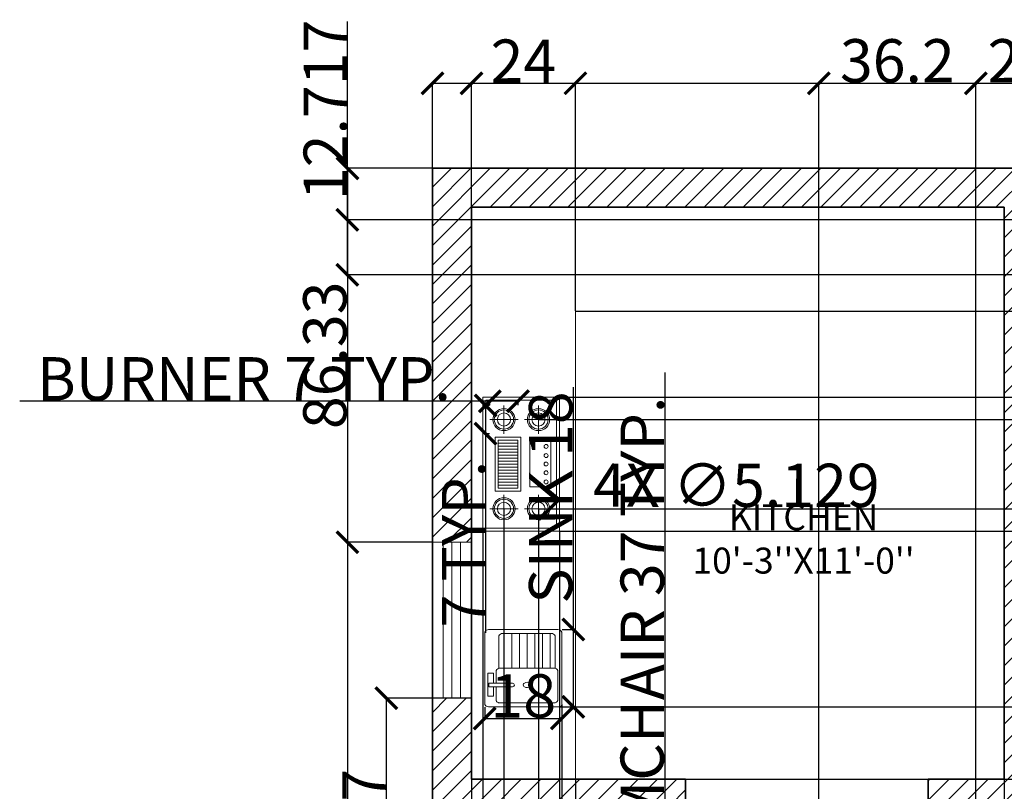
# Model space of a CAD drawing. Units: inches. Extents: x 90933 to 91345, y 21207 to 21646.
# Tile 3 of 4: x 90933 to 91160, y 21458 to 21636. Entities that reach past the tile are written whole.
import ezdxf

# ---------------------------------------------------------------- set-up
doc = ezdxf.new("R2010")
doc.units = ezdxf.units.IN
for name, color, linetype, lineweight in [('A-ANNO-DIMS', 2, 'Continuous', 18), ('A-AREA-IDEN', 7, 'Continuous', 25), ('A-EQPM', 9, 'Continuous', 18), ('A-EQPM-PATT', 9, 'Continuous', 13), ('A-FLOR-CASE', 42, 'Continuous', 18), ('A-FLOR-FIXT', 9, 'Continuous', 18), ('A-WALL-PATT', 8, 'Continuous', 13), ('Walls', 7, 'Continuous', 35), ('Windows', 140, 'Continuous', 18)]:
    doc.layers.add(name, color=color, linetype=linetype, lineweight=lineweight)
doc.styles.get("Standard").update_dxf_attribs({"font": 'arial.ttf'})
doc.dimstyles.get("Standard").update_dxf_attribs({"dimtxt": 10, "dimasz": 5, "dimexe": 0.18, "dimexo": 0.0625, "dimgap": 0.09, "dimtad": 1, "dimdec": 1, "dimzin": 0, "dimdsep": 46, "dimlunit": 4, "dimtxsty": 'Standard', "dimblk": 'ARCHTICK', "dimcen": 0.09, "dimadec": 0, "dimazin": 0, "dimtfac": 1, "dimtdec": 1, "dimtofl": 0, "dimtmove": 0, "dimatfit": 3, "dimldrblk": 'NONE', "dimfxl": 1, "dimtolj": 1, "dimtzin": 0, "dimarcsym": 0})

# ---------------------------------------------------------------- blocks, each defined once
blk = doc.blocks.new('S_SINK12')
for p, q in [((0.25, 0.45), (0.25, 0)), ((0.35, 0.45), (0.35, 0)), ((0.45, 0.45), (0.45, 0)), ((0.55, 0.45), (0.55, 0)), ((0.65, 0.45), (0.65, 0)), ((0.75, 0.45), (0.75, 0)), ((0.85, 0.45), (0.85, 0))]:
    blk.add_line(p, q)
for points in [[(0, -0.469), (0, 0.469, -0.310961), (0.05, 0.5), (0.95, 0.5, -0.310466), (1, 0.469), (1, -0.469, -0.414214), (0.969, -0.5), (0.05, -0.5, -0.309971)], [(0.052, -0.195), (0.052, -0.242), (0.362, -0.242, 1), (0.362, -0.195)], [(0.5, -0.217), (0.503, -0.229, 0.107136), (0.516, -0.241, 0.076468), (0.534, -0.249), (0.554, -0.251), (0.575, -0.248, 0.076468), (0.592, -0.241, 0.107136), (0.604, -0.229), (0.608, -0.217), (0.604, -0.205, 0.107136), (0.592, -0.193, 0.076468), (0.575, -0.186), (0.554, -0.183), (0.532, -0.186, 0.076468), (0.516, -0.193, 0.107136), (0.503, -0.205)]]:
    blk.add_lwpolyline(points, format="xyb", close=True)
for points in [[(0.185, -0.001), (0.185, 0.419, -0.310466), (0.235, 0.45), (0.862, 0.45, -0.310466), (0.912, 0.419), (0.912, 0, -0.310466)], [(0.15, -0.195), (0.15, -0.031, -0.310466), (0.2, 0), (0.9, 0, -0.310466), (0.95, -0.031), (0.95, -0.419, -0.310466), (0.9, -0.45), (0.2, -0.45), (0.18, -0.448, -0.071009), (0.165, -0.442, -0.106323), (0.153, -0.432), (0.15, -0.422), (0.151, -0.419)]]:
    blk.add_lwpolyline(points, format="xyb")
for points in [[(0.114, -0.242), (0.114, -0.364), (0.039, -0.364), (0.039, -0.064), (0.114, -0.064), (0.114, -0.195)], [(0.15, -0.419), (0.15, -0.242)]]:
    blk.add_lwpolyline(points)
blk = doc.blocks.new('COOKTOP-BURNER')
for p, q in [((0, -3.26), (0, 3.26)), ((3.26, 0), (-3.26, 0))]:
    blk.add_line(p, q)
for radius in [2.56, 2.22, 1.52]:
    blk.add_circle((0, 0), radius)
blk = doc.blocks.new('WINDOW-GLAZING-36IN')
for p, q in [((0, 4), (36, 4)), ((0, 2), (36, 2)), ((0, 0), (36, 0))]:
    blk.add_line(p, q)
blk = doc.blocks.new('_ArchTick')
at = {"color": 0, "linetype": 'ByBlock', "const_width": 0.15}
blk.add_lwpolyline([(-0.5, -0.5), (0.5, 0.5)], dxfattribs=at)
blk = doc.blocks.new('*D18')
at = {"layer": 'A-ANNO-DIMS', "color": 0, "lineweight": -2, "transparency": 16777216}
for p, q in [((91041.35, 21547.85), (90932.83, 21547.85)), ((91041.35, 21546.93), (91041.35, 21548.03)), ((91047.87, 21547.85), (91041.35, 21547.85)), ((91047.87, 21546.93), (91047.87, 21548.03))]:
    blk.add_line(p, q, dxfattribs=at)
at = {"layer": 'Defpoints', "color": 0, "transparency": 16777216}
for p in [(91041.35, 21547.85), (91041.35, 21546.87), (91047.87, 21546.87)]:
    blk.add_point(p, dxfattribs=at)
at = {"layer": 'A-ANNO-DIMS', "color": 0, "lineweight": -2, "transparency": 16777216, "xscale": 5, "yscale": 5, "zscale": 5, "rotation": 180}
blk.add_blockref('_ArchTick', (91041.35, 21547.85), dxfattribs=at)
at = {"layer": 'A-ANNO-DIMS', "color": 0, "lineweight": -2, "transparency": 16777216, "xscale": 5, "yscale": 5, "zscale": 5}
blk.add_blockref('_ArchTick', (91047.87, 21547.85), dxfattribs=at)
at = {"layer": 'A-ANNO-DIMS', "color": 0, "transparency": 16777216, "insert": (90984.59, 21553.02), "char_height": 10, "attachment_point": 5}
blk.add_mtext('\\A1;BURNER 7 TYP.', dxfattribs=at)
blk = doc.blocks.new('_None')
blk = doc.blocks.new('*D19')
at = {"layer": 'A-ANNO-DIMS', "color": 0, "lineweight": -2, "transparency": 16777216}
for p, q in [((91041.29, 21546.87), (91040.19, 21546.87)), ((91040.37, 21546.87), (91040.37, 21540.35)), ((91041.29, 21540.35), (91040.19, 21540.35)), ((91040.37, 21540.35), (91040.37, 21494.35))]:
    blk.add_line(p, q, dxfattribs=at)
at = {"layer": 'Defpoints', "color": 0, "transparency": 16777216}
for p in [(91041.35, 21546.87), (91040.37, 21540.35), (91041.35, 21540.35)]:
    blk.add_point(p, dxfattribs=at)
at = {"layer": 'A-ANNO-DIMS', "color": 0, "lineweight": -2, "transparency": 16777216, "xscale": 5, "yscale": 5, "zscale": 5}
for p, rotation in [((91040.37, 21546.87), 90), ((91040.37, 21540.35), 270)]:
    blk.add_blockref('_ArchTick', p, dxfattribs=dict(at, rotation=rotation))
at = {"layer": 'A-ANNO-DIMS', "color": 0, "transparency": 16777216, "insert": (91035.28, 21514.85), "char_height": 10, "attachment_point": 5, "rotation": 90}
blk.add_mtext('\\A1;7 TYP.', dxfattribs=at)
blk = doc.blocks.new('*D24')
at = {"layer": 'A-ANNO-DIMS', "color": 0, "lineweight": -2, "transparency": 16777216}
for p, q in [((91081.79, 21421.63), (91081.79, 21554.45)), ((91076.29, 21421.63), (91081.97, 21421.63)), ((91081.79, 21384.54), (91081.79, 21421.63)), ((91076.29, 21384.54), (91081.97, 21384.54))]:
    blk.add_line(p, q, dxfattribs=at)
at = {"layer": 'Defpoints', "color": 0, "transparency": 16777216}
for p in [(91076.22, 21421.63), (91081.79, 21421.63), (91076.22, 21384.54)]:
    blk.add_point(p, dxfattribs=at)
at = {"layer": 'A-ANNO-DIMS', "color": 0, "lineweight": -2, "transparency": 16777216, "xscale": 5, "yscale": 5, "zscale": 5}
for p, rotation in [((91081.79, 21421.63), 90), ((91081.79, 21384.54), 270)]:
    blk.add_blockref('_ArchTick', p, dxfattribs=dict(at, rotation=rotation))
at = {"layer": 'A-ANNO-DIMS', "color": 0, "transparency": 16777216, "insert": (91076.52, 21490.54), "char_height": 10, "attachment_point": 5, "rotation": 90}
blk.add_mtext('\\A1;ARMCHAIR 37 TYP.', dxfattribs=at)
blk = doc.blocks.new('*D34')
at = {"layer": 'A-ANNO-DIMS', "color": 0, "lineweight": -2, "transparency": 16777216}
for p, q in [((91060.64, 21495.13), (91060.64, 21551.09)), ((91058.03, 21495.13), (91060.82, 21495.13)), ((91060.64, 21477.3), (91060.64, 21495.13)), ((91058.03, 21477.3), (91060.82, 21477.3))]:
    blk.add_line(p, q, dxfattribs=at)
at = {"layer": 'Defpoints', "color": 0, "transparency": 16777216}
for p in [(91057.97, 21495.13), (91060.64, 21495.13), (91057.97, 21477.3)]:
    blk.add_point(p, dxfattribs=at)
at = {"layer": 'A-ANNO-DIMS', "color": 0, "lineweight": -2, "transparency": 16777216, "xscale": 5, "yscale": 5, "zscale": 5}
for p, rotation in [((91060.64, 21495.13), 90), ((91060.64, 21477.3), 270)]:
    blk.add_blockref('_ArchTick', p, dxfattribs=dict(at, rotation=rotation))
at = {"layer": 'A-ANNO-DIMS', "color": 0, "transparency": 16777216, "insert": (91055.38, 21525.61), "char_height": 10, "attachment_point": 5, "rotation": 90}
blk.add_mtext('\\A1;SINK 18', dxfattribs=at)
blk = doc.blocks.new('*D35')
at = {"layer": 'A-ANNO-DIMS', "color": 0, "lineweight": -2, "transparency": 16777216}
for p, q in [((91040.17, 21477.23), (91040.17, 21474.44)), ((91057.97, 21477.23), (91057.97, 21474.44)), ((91040.17, 21474.62), (91057.97, 21474.62))]:
    blk.add_line(p, q, dxfattribs=at)
at = {"layer": 'Defpoints', "color": 0, "transparency": 16777216}
for p in [(91040.17, 21477.3), (91057.97, 21477.3), (91057.97, 21474.62)]:
    blk.add_point(p, dxfattribs=at)
at = {"layer": 'A-ANNO-DIMS', "color": 0, "lineweight": -2, "transparency": 16777216, "xscale": 5, "yscale": 5, "zscale": 5, "rotation": 180}
blk.add_blockref('_ArchTick', (91040.17, 21474.62), dxfattribs=at)
at = {"layer": 'A-ANNO-DIMS', "color": 0, "lineweight": -2, "transparency": 16777216, "xscale": 5, "yscale": 5, "zscale": 5}
blk.add_blockref('_ArchTick', (91057.97, 21474.62), dxfattribs=at)
at = {"layer": 'A-ANNO-DIMS', "color": 0, "transparency": 16777216, "insert": (91049.07, 21479.82), "char_height": 10, "attachment_point": 5}
blk.add_mtext('\\A1;18', dxfattribs=at)
blk = doc.blocks.new('*D42')
at = {"layer": 'A-ANNO-DIMS', "color": 0, "lineweight": -2, "transparency": 16777216}
for p, q in [((91028.04, 21601.62), (91008.29, 21601.62)), ((91008.47, 21601.62), (91008.47, 21515.28)), ((91028.04, 21515.28), (91008.29, 21515.28))]:
    blk.add_line(p, q, dxfattribs=at)
at = {"layer": 'Defpoints', "color": 0, "transparency": 16777216}
for p in [(91028.1, 21601.62), (91008.47, 21515.28), (91028.1, 21515.28)]:
    blk.add_point(p, dxfattribs=at)
at = {"layer": 'A-ANNO-DIMS', "color": 0, "lineweight": -2, "transparency": 16777216, "xscale": 5, "yscale": 5, "zscale": 5}
for p, rotation in [((91008.47, 21601.62), 90), ((91008.47, 21515.28), 270)]:
    blk.add_blockref('_ArchTick', p, dxfattribs=dict(at, rotation=rotation))
at = {"layer": 'A-ANNO-DIMS', "color": 0, "transparency": 16777216, "insert": (91003.27, 21558.45), "char_height": 10, "attachment_point": 5, "rotation": 90}
blk.add_mtext('\\A1;86.33', dxfattribs=at)
blk = doc.blocks.new('*D43')
at = {"layer": 'A-ANNO-DIMS', "color": 0, "lineweight": -2, "transparency": 16777216}
for p, q in [((91037.04, 21479.28), (91017.29, 21479.28)), ((91017.47, 21412.62), (91017.47, 21479.28)), ((91037.04, 21412.62), (91017.29, 21412.62))]:
    blk.add_line(p, q, dxfattribs=at)
at = {"layer": 'Defpoints', "color": 0, "transparency": 16777216}
for p in [(91017.47, 21479.28), (91037.1, 21479.28), (91037.1, 21412.62)]:
    blk.add_point(p, dxfattribs=at)
at = {"layer": 'A-ANNO-DIMS', "color": 0, "lineweight": -2, "transparency": 16777216, "xscale": 5, "yscale": 5, "zscale": 5}
for p, rotation in [((91017.47, 21479.28), 90), ((91017.47, 21412.62), 270)]:
    blk.add_blockref('_ArchTick', p, dxfattribs=dict(at, rotation=rotation))
at = {"layer": 'A-ANNO-DIMS', "color": 0, "transparency": 16777216, "insert": (91012.27, 21445.95), "char_height": 10, "attachment_point": 5, "rotation": 90}
blk.add_mtext('\\A1;66.67', dxfattribs=at)
blk = doc.blocks.new('*D49')
at = {"layer": 'A-ANNO-DIMS', "color": 0, "lineweight": -2, "transparency": 16777216}
for p, q in [((91160.1, 21460.55), (91160.1, 21209.81)), ((91142.5, 21454.55), (91142.5, 21209.81)), ((91142.5, 21209.99), (91160.1, 21209.99)), ((91160.1, 21209.99), (91205.85, 21209.99))]:
    blk.add_line(p, q, dxfattribs=at)
at = {"layer": 'Defpoints', "color": 0, "transparency": 16777216}
for p in [(91160.1, 21460.62), (91142.5, 21454.62), (91160.1, 21209.99)]:
    blk.add_point(p, dxfattribs=at)
at = {"layer": 'A-ANNO-DIMS', "color": 0, "lineweight": -2, "transparency": 16777216, "xscale": 5, "yscale": 5, "zscale": 5, "rotation": 180}
blk.add_blockref('_ArchTick', (91142.5, 21209.99), dxfattribs=at)
at = {"layer": 'A-ANNO-DIMS', "color": 0, "lineweight": -2, "transparency": 16777216, "xscale": 5, "yscale": 5, "zscale": 5}
blk.add_blockref('_ArchTick', (91160.1, 21209.99), dxfattribs=at)
at = {"layer": 'A-ANNO-DIMS', "color": 0, "transparency": 16777216, "insert": (91185.47, 21215.18), "char_height": 10, "attachment_point": 5}
blk.add_mtext('\\A1;17.596', dxfattribs=at)
blk = doc.blocks.new('*D52')
at = {"layer": 'A-ANNO-DIMS', "color": 0, "lineweight": -2, "transparency": 16777216}
for p, q in [((91037.1, 21592.68), (91037.1, 21621.43)), ((91037.1, 21621.25), (91061.1, 21621.25)), ((91061.1, 21568.68), (91061.1, 21621.43))]:
    blk.add_line(p, q, dxfattribs=at)
at = {"layer": 'Defpoints', "color": 0, "transparency": 16777216}
for p in [(91061.1, 21621.25), (91037.1, 21592.62), (91061.1, 21568.62)]:
    blk.add_point(p, dxfattribs=at)
at = {"layer": 'A-ANNO-DIMS', "color": 0, "lineweight": -2, "transparency": 16777216, "xscale": 5, "yscale": 5, "zscale": 5, "rotation": 180}
blk.add_blockref('_ArchTick', (91037.1, 21621.25), dxfattribs=at)
at = {"layer": 'A-ANNO-DIMS', "color": 0, "lineweight": -2, "transparency": 16777216, "xscale": 5, "yscale": 5, "zscale": 5}
blk.add_blockref('_ArchTick', (91061.1, 21621.25), dxfattribs=at)
at = {"layer": 'A-ANNO-DIMS', "color": 0, "transparency": 16777216, "insert": (91049.1, 21626.36), "char_height": 10, "attachment_point": 5}
blk.add_mtext('\\A1;24', dxfattribs=at)
blk = doc.blocks.new('*D53')
at = {"layer": 'A-ANNO-DIMS', "color": 0, "lineweight": -2, "transparency": 16777216}
for p, q in [((91160.1, 21460.55), (91160.1, 21209.81)), ((91166.1, 21460.55), (91166.1, 21209.81)), ((91160.1, 21209.99), (91166.1, 21209.99)), ((91166.1, 21209.99), (91177.88, 21209.99))]:
    blk.add_line(p, q, dxfattribs=at)
at = {"layer": 'Defpoints', "color": 0, "transparency": 16777216}
for p in [(91160.1, 21460.62), (91166.1, 21460.62), (91166.1, 21209.99)]:
    blk.add_point(p, dxfattribs=at)
at = {"layer": 'A-ANNO-DIMS', "color": 0, "lineweight": -2, "transparency": 16777216, "xscale": 5, "yscale": 5, "zscale": 5, "rotation": 180}
blk.add_blockref('_ArchTick', (91160.1, 21209.99), dxfattribs=at)
at = {"layer": 'A-ANNO-DIMS', "color": 0, "lineweight": -2, "transparency": 16777216, "xscale": 5, "yscale": 5, "zscale": 5}
blk.add_blockref('_ArchTick', (91166.1, 21209.99), dxfattribs=at)
at = {"layer": 'A-ANNO-DIMS', "color": 0, "transparency": 16777216, "insert": (91174.49, 21215.18), "char_height": 10, "attachment_point": 5}
blk.add_mtext('\\A1;6', dxfattribs=at)
blk = doc.blocks.new('*D58')
at = {"layer": 'A-ANNO-DIMS', "color": 0, "lineweight": -2, "transparency": 16777216}
for p, q in [((91039.71, 21517.79), (91039.71, 21209.81)), ((91057.43, 21517.79), (91057.43, 21209.81)), ((91039.71, 21209.99), (91057.43, 21209.99)), ((91057.43, 21209.99), (91103.17, 21209.99))]:
    blk.add_line(p, q, dxfattribs=at)
at = {"layer": 'Defpoints', "color": 0, "transparency": 16777216}
for p in [(91039.71, 21517.85), (91057.43, 21517.85), (91057.43, 21209.99)]:
    blk.add_point(p, dxfattribs=at)
at = {"layer": 'A-ANNO-DIMS', "color": 0, "lineweight": -2, "transparency": 16777216, "xscale": 5, "yscale": 5, "zscale": 5, "rotation": 180}
blk.add_blockref('_ArchTick', (91039.71, 21209.99), dxfattribs=at)
at = {"layer": 'A-ANNO-DIMS', "color": 0, "lineweight": -2, "transparency": 16777216, "xscale": 5, "yscale": 5, "zscale": 5}
blk.add_blockref('_ArchTick', (91057.43, 21209.99), dxfattribs=at)
at = {"layer": 'A-ANNO-DIMS', "color": 0, "transparency": 16777216, "insert": (91082.8, 21215.18), "char_height": 10, "attachment_point": 5}
blk.add_mtext('\\A1;17.716', dxfattribs=at)
blk = doc.blocks.new('*D59')
at = {"layer": 'A-ANNO-DIMS', "color": 0, "lineweight": -2, "transparency": 16777216}
for p, q in [((91326.73, 21548.77), (91326.73, 21595.45)), ((91057.49, 21548.77), (91326.91, 21548.77)), ((91326.73, 21517.85), (91326.73, 21548.77)), ((91057.49, 21517.85), (91326.91, 21517.85))]:
    blk.add_line(p, q, dxfattribs=at)
at = {"layer": 'Defpoints', "color": 0, "transparency": 16777216}
for p in [(91057.43, 21548.77), (91326.73, 21548.77), (91057.43, 21517.85)]:
    blk.add_point(p, dxfattribs=at)
at = {"layer": 'A-ANNO-DIMS', "color": 0, "lineweight": -2, "transparency": 16777216, "xscale": 5, "yscale": 5, "zscale": 5}
for p, rotation in [((91326.73, 21548.77), 90), ((91326.73, 21517.85), 270)]:
    blk.add_blockref('_ArchTick', p, dxfattribs=dict(at, rotation=rotation))
at = {"layer": 'A-ANNO-DIMS', "color": 0, "transparency": 16777216, "insert": (91321.53, 21574.61), "char_height": 10, "attachment_point": 5, "rotation": 90}
blk.add_mtext('\\A1;30.916', dxfattribs=at)
blk = doc.blocks.new('*D60')
at = {"layer": 'A-ANNO-DIMS', "color": 0, "lineweight": -2, "transparency": 16777216}
for p, q in [((91117.31, 21395.74), (91117.31, 21621.43)), ((91117.31, 21621.25), (91153.51, 21621.25)), ((91153.51, 21395.74), (91153.51, 21621.43))]:
    blk.add_line(p, q, dxfattribs=at)
at = {"layer": 'Defpoints', "color": 0, "transparency": 16777216}
for p in [(91153.51, 21621.25), (91117.31, 21395.68), (91153.51, 21395.68)]:
    blk.add_point(p, dxfattribs=at)
at = {"layer": 'A-ANNO-DIMS', "color": 0, "lineweight": -2, "transparency": 16777216, "xscale": 5, "yscale": 5, "zscale": 5, "rotation": 180}
blk.add_blockref('_ArchTick', (91117.31, 21621.25), dxfattribs=at)
at = {"layer": 'A-ANNO-DIMS', "color": 0, "lineweight": -2, "transparency": 16777216, "xscale": 5, "yscale": 5, "zscale": 5}
blk.add_blockref('_ArchTick', (91153.51, 21621.25), dxfattribs=at)
at = {"layer": 'A-ANNO-DIMS', "color": 0, "transparency": 16777216, "insert": (91135.41, 21626.44), "char_height": 10, "attachment_point": 5}
blk.add_mtext('\\A1;36.2', dxfattribs=at)
blk = doc.blocks.new('*D63')
at = {"layer": 'A-ANNO-DIMS', "color": 0, "lineweight": -2, "transparency": 16777216}
for p, q in [((91008.47, 21589.73), (91008.47, 21635.49)), ((91252.43, 21589.73), (91008.29, 21589.73)), ((91008.47, 21577.01), (91008.47, 21589.73)), ((91252.43, 21577.01), (91008.29, 21577.01))]:
    blk.add_line(p, q, dxfattribs=at)
at = {"layer": 'Defpoints', "color": 0, "transparency": 16777216}
for p in [(91008.47, 21589.73), (91252.49, 21589.73), (91252.49, 21577.01)]:
    blk.add_point(p, dxfattribs=at)
at = {"layer": 'A-ANNO-DIMS', "color": 0, "lineweight": -2, "transparency": 16777216, "xscale": 5, "yscale": 5, "zscale": 5}
for p, rotation in [((91008.47, 21589.73), 90), ((91008.47, 21577.01), 270)]:
    blk.add_blockref('_ArchTick', p, dxfattribs=dict(at, rotation=rotation))
at = {"layer": 'A-ANNO-DIMS', "color": 0, "transparency": 16777216, "insert": (91003.36, 21615.11), "char_height": 10, "attachment_point": 5, "rotation": 90}
blk.add_mtext('\\A1;12.717', dxfattribs=at)
blk = doc.blocks.new('*D64')
at = {"layer": 'A-ANNO-DIMS', "color": 0, "lineweight": -2, "transparency": 16777216}
for p, q in [((91028.1, 21601.68), (91028.1, 21621.43)), ((91028.1, 21621.25), (91307.1, 21621.25)), ((91307.1, 21601.68), (91307.1, 21621.43))]:
    blk.add_line(p, q, dxfattribs=at)
at = {"layer": 'Defpoints', "color": 0, "transparency": 16777216}
for p in [(91307.1, 21621.25), (91028.1, 21601.62), (91307.1, 21601.62)]:
    blk.add_point(p, dxfattribs=at)
at = {"layer": 'A-ANNO-DIMS', "color": 0, "lineweight": -2, "transparency": 16777216, "xscale": 5, "yscale": 5, "zscale": 5, "rotation": 180}
blk.add_blockref('_ArchTick', (91028.1, 21621.25), dxfattribs=at)
at = {"layer": 'A-ANNO-DIMS', "color": 0, "lineweight": -2, "transparency": 16777216, "xscale": 5, "yscale": 5, "zscale": 5}
blk.add_blockref('_ArchTick', (91307.1, 21621.25), dxfattribs=at)
at = {"layer": 'A-ANNO-DIMS', "color": 0, "transparency": 16777216, "insert": (91167.6, 21626.44), "char_height": 10, "attachment_point": 5}
blk.add_mtext('\\A1;279', dxfattribs=at)
blk = doc.blocks.new('*D65')
at = {"layer": 'A-ANNO-DIMS', "color": 0, "lineweight": -2, "transparency": 16777216}
for p, q in [((91028.04, 21601.62), (91008.29, 21601.62)), ((91008.47, 21601.62), (91008.47, 21229.62)), ((91028.04, 21229.62), (91008.29, 21229.62))]:
    blk.add_line(p, q, dxfattribs=at)
at = {"layer": 'Defpoints', "color": 0, "transparency": 16777216}
for p in [(91028.1, 21601.62), (91008.47, 21229.62), (91028.1, 21229.62)]:
    blk.add_point(p, dxfattribs=at)
at = {"layer": 'A-ANNO-DIMS', "color": 0, "lineweight": -2, "transparency": 16777216, "xscale": 5, "yscale": 5, "zscale": 5}
for p, rotation in [((91008.47, 21601.62), 90), ((91008.47, 21229.62), 270)]:
    blk.add_blockref('_ArchTick', p, dxfattribs=dict(at, rotation=rotation))
at = {"layer": 'A-ANNO-DIMS', "color": 0, "transparency": 16777216, "insert": (91003.27, 21415.62), "char_height": 10, "attachment_point": 5, "rotation": 90}
blk.add_mtext('\\A1;372', dxfattribs=at)
blk = doc.blocks.new('*D66')
at = {"layer": 'A-ANNO-DIMS', "color": 0, "lineweight": -2, "transparency": 16777216}
for p, q in [((91061.16, 21568.62), (91326.91, 21568.62)), ((91326.73, 21568.62), (91326.73, 21548.77)), ((91057.49, 21548.77), (91326.91, 21548.77)), ((91326.73, 21548.77), (91326.73, 21503.02))]:
    blk.add_line(p, q, dxfattribs=at)
at = {"layer": 'Defpoints', "color": 0, "transparency": 16777216}
for p in [(91061.1, 21568.62), (91057.43, 21548.77), (91326.73, 21548.77)]:
    blk.add_point(p, dxfattribs=at)
at = {"layer": 'A-ANNO-DIMS', "color": 0, "lineweight": -2, "transparency": 16777216, "xscale": 5, "yscale": 5, "zscale": 5}
for p, rotation in [((91326.73, 21568.62), 90), ((91326.73, 21548.77), 270)]:
    blk.add_blockref('_ArchTick', p, dxfattribs=dict(at, rotation=rotation))
at = {"layer": 'A-ANNO-DIMS', "color": 0, "transparency": 16777216, "insert": (91321.53, 21523.4), "char_height": 10, "attachment_point": 5, "rotation": 90}
blk.add_mtext('\\A1;19.846', dxfattribs=at)
blk = doc.blocks.new('*D67')
at = {"layer": 'A-ANNO-DIMS', "color": 0, "lineweight": -2, "transparency": 16777216}
for p, q in [((91326.73, 21477.31), (91326.73, 21507.53)), ((91057.47, 21477.31), (91326.91, 21477.31)), ((91326.73, 21460.62), (91326.73, 21477.31)), ((91061.16, 21460.62), (91326.91, 21460.62))]:
    blk.add_line(p, q, dxfattribs=at)
at = {"layer": 'Defpoints', "color": 0, "transparency": 16777216}
for p in [(91057.41, 21477.31), (91326.73, 21477.31), (91061.1, 21460.62)]:
    blk.add_point(p, dxfattribs=at)
at = {"layer": 'A-ANNO-DIMS', "color": 0, "lineweight": -2, "transparency": 16777216, "xscale": 5, "yscale": 5, "zscale": 5}
for p, rotation in [((91326.73, 21477.31), 90), ((91326.73, 21460.62), 270)]:
    blk.add_blockref('_ArchTick', p, dxfattribs=dict(at, rotation=rotation))
at = {"layer": 'A-ANNO-DIMS', "color": 0, "transparency": 16777216, "insert": (91321.53, 21494.92), "char_height": 10, "attachment_point": 5, "rotation": 90}
blk.add_mtext('\\A1;16.7', dxfattribs=at)
blk = doc.blocks.new('*D71')
at = {"layer": 'A-ANNO-DIMS', "color": 0, "lineweight": -2, "transparency": 16777216}
for p, q in [((91044.61, 21522.95), (91044.61, 21209.81)), ((91052.59, 21522.95), (91052.59, 21209.81)), ((91044.61, 21209.99), (91052.59, 21209.99)), ((91052.59, 21209.99), (91083.68, 21209.99))]:
    blk.add_line(p, q, dxfattribs=at)
at = {"layer": 'Defpoints', "color": 0, "transparency": 16777216}
for p in [(91044.61, 21523.01), (91052.59, 21523.01), (91052.59, 21209.99)]:
    blk.add_point(p, dxfattribs=at)
at = {"layer": 'A-ANNO-DIMS', "color": 0, "lineweight": -2, "transparency": 16777216, "xscale": 5, "yscale": 5, "zscale": 5, "rotation": 180}
blk.add_blockref('_ArchTick', (91044.61, 21209.99), dxfattribs=at)
at = {"layer": 'A-ANNO-DIMS', "color": 0, "lineweight": -2, "transparency": 16777216, "xscale": 5, "yscale": 5, "zscale": 5}
blk.add_blockref('_ArchTick', (91052.59, 21209.99), dxfattribs=at)
at = {"layer": 'A-ANNO-DIMS', "color": 0, "transparency": 16777216, "insert": (91070.64, 21215.18), "char_height": 10, "attachment_point": 5}
blk.add_mtext('\\A1;7.98', dxfattribs=at)
blk = doc.blocks.new('*D72')
at = {"layer": 'A-ANNO-DIMS', "color": 0, "lineweight": -2, "transparency": 16777216}
for p, q in [((91326.73, 21543.61), (91326.73, 21590.47)), ((91052.65, 21543.61), (91326.91, 21543.61)), ((91326.73, 21523.01), (91326.73, 21543.61)), ((91052.65, 21523.01), (91326.91, 21523.01))]:
    blk.add_line(p, q, dxfattribs=at)
at = {"layer": 'Defpoints', "color": 0, "transparency": 16777216}
for p in [(91052.59, 21543.61), (91326.73, 21543.61), (91052.59, 21523.01)]:
    blk.add_point(p, dxfattribs=at)
at = {"layer": 'A-ANNO-DIMS', "color": 0, "lineweight": -2, "transparency": 16777216, "xscale": 5, "yscale": 5, "zscale": 5}
for p, rotation in [((91326.73, 21543.61), 90), ((91326.73, 21523.01), 270)]:
    blk.add_blockref('_ArchTick', p, dxfattribs=dict(at, rotation=rotation))
at = {"layer": 'A-ANNO-DIMS', "color": 0, "transparency": 16777216, "insert": (91321.53, 21569.54), "char_height": 10, "attachment_point": 5, "rotation": 90}
blk.add_mtext('\\A1;20.597', dxfattribs=at)
blk = doc.blocks.new('*D73')
at = {"layer": 'A-ANNO-DIMS', "color": 0, "lineweight": -2, "transparency": 16777216}
for p, q in [((91039.71, 21517.79), (91039.71, 21209.81)), ((91037.1, 21515.22), (91037.1, 21209.81)), ((91037.1, 21209.99), (91039.71, 21209.99)), ((91039.71, 21209.99), (91069.11, 21209.99))]:
    blk.add_line(p, q, dxfattribs=at)
at = {"layer": 'Defpoints', "color": 0, "transparency": 16777216}
for p in [(91039.71, 21517.85), (91037.1, 21515.28), (91039.71, 21209.99)]:
    blk.add_point(p, dxfattribs=at)
at = {"layer": 'A-ANNO-DIMS', "color": 0, "lineweight": -2, "transparency": 16777216, "xscale": 5, "yscale": 5, "zscale": 5, "rotation": 180}
blk.add_blockref('_ArchTick', (91037.1, 21209.99), dxfattribs=at)
at = {"layer": 'A-ANNO-DIMS', "color": 0, "lineweight": -2, "transparency": 16777216, "xscale": 5, "yscale": 5, "zscale": 5}
blk.add_blockref('_ArchTick', (91039.71, 21209.99), dxfattribs=at)
at = {"layer": 'A-ANNO-DIMS', "color": 0, "transparency": 16777216, "insert": (91056.91, 21215.18), "char_height": 10, "attachment_point": 5}
blk.add_mtext('\\A1;2.61', dxfattribs=at)
blk = doc.blocks.new('*D74')
at = {"layer": 'A-ANNO-DIMS', "color": 0, "lineweight": -2, "transparency": 16777216}
for p, q in [((91057.97, 21477.81), (91057.97, 21209.81)), ((91061.1, 21460.55), (91061.1, 21209.81)), ((91057.97, 21209.99), (91019.09, 21209.99)), ((91061.1, 21209.99), (91057.97, 21209.99))]:
    blk.add_line(p, q, dxfattribs=at)
at = {"layer": 'Defpoints', "color": 0, "transparency": 16777216}
for p in [(91057.97, 21477.87), (91061.1, 21460.62), (91057.97, 21209.99)]:
    blk.add_point(p, dxfattribs=at)
at = {"layer": 'A-ANNO-DIMS', "color": 0, "lineweight": -2, "transparency": 16777216, "xscale": 5, "yscale": 5, "zscale": 5, "rotation": 180}
blk.add_blockref('_ArchTick', (91057.97, 21209.99), dxfattribs=at)
at = {"layer": 'A-ANNO-DIMS', "color": 0, "lineweight": -2, "transparency": 16777216, "xscale": 5, "yscale": 5, "zscale": 5}
blk.add_blockref('_ArchTick', (91061.1, 21209.99), dxfattribs=at)
at = {"layer": 'A-ANNO-DIMS', "color": 0, "transparency": 16777216, "insert": (91036.03, 21215.18), "char_height": 10, "attachment_point": 5}
blk.add_mtext('\\A1;3.134', dxfattribs=at)
blk = doc.blocks.new('*D78')
at = {"layer": 'A-ANNO-DIMS', "color": 0, "lineweight": -2, "transparency": 16777216}
for p, q in [((91052.5, 21523.01), (91052.68, 21523.01)), ((91052.59, 21522.92), (91052.59, 21523.1)), ((91131.34, 21522.93), (91055.15, 21523.01))]:
    blk.add_line(p, q, dxfattribs=at)
at = {"layer": 'Defpoints', "color": 0, "transparency": 16777216}
for p in [(91050.02, 21523.02), (91055.15, 21523.01)]:
    blk.add_point(p, dxfattribs=at)
at = {"layer": 'A-ANNO-DIMS', "color": 0, "lineweight": -2, "transparency": 16777216, "xscale": 5, "yscale": 5, "zscale": 5, "rotation": 179.9410859933045}
blk.add_blockref('_ArchTick', (91055.15, 21523.01), dxfattribs=at)
at = {"layer": 'A-ANNO-DIMS', "color": 0, "transparency": 16777216, "insert": (91098.25, 21528.44), "char_height": 10, "attachment_point": 5, "rotation": 359.9411}
blk.add_mtext('\\A1;4X ∅5.129', dxfattribs=at)

msp = doc.modelspace()

# ---------------------------------------------------------------- hatches: boundary and pattern name
at = {"layer": 'A-EQPM-PATT'}
h = msp.add_hatch(dxfattribs=at)
h.set_pattern_fill('ANSI31', color=256, scale=0.218814173, angle=-45, style=0)
h.paths.add_polyline_path([(91043.2566, 21527.7535), (91047.8397, 21527.7535), (91047.8397, 21538.8692), (91043.2566, 21538.8692)])
at = {"layer": 'A-WALL-PATT', "transparency": 33554585}
h = msp.add_hatch(dxfattribs=at)
h.set_pattern_fill('ANSI31', color=256)
h.paths.add_polyline_path([(91179.1445, 21601.6157), (91028.1004, 21601.6157), (91028.1004, 21515.2814), (91037.1004, 21515.2814), (91037.1004, 21592.6157), (91160.1004, 21592.6157), (91160.1004, 21460.6157), (91142.5048, 21460.6157), (91142.5048, 21454.6157), (91175.976, 21454.6157), (91175.976, 21460.6157), (91166.1004, 21460.6157), (91166.1004, 21592.6157), (91179.1445, 21592.6157)])
h.paths.add_polyline_path([(91307.1004, 21601.6157), (91215.1445, 21601.6157), (91215.1445, 21592.6157), (91298.1004, 21592.6157), (91298.1004, 21460.6157), (91272.1605, 21460.6157), (91272.1605, 21454.6157), (91298.1004, 21454.6157), (91298.1004, 21384.4519), (91307.1004, 21384.4519)])
h.paths.add_polyline_path([(91037.1004, 21454.6157), (91086.5447, 21454.6157), (91086.5447, 21460.6157), (91037.1004, 21460.6157), (91037.1004, 21479.2814), (91028.1004, 21479.2814), (91028.1004, 21412.6157), (91037.1004, 21412.6157)])
h.paths.add_polyline_path([(91307.1004, 21348.4519), (91298.1004, 21348.4519), (91298.1004, 21322.6157), (91244.1004, 21322.6157), (91244.1004, 21454.6157), (91246.6116, 21454.6157), (91246.6116, 21460.6157), (91201.4342, 21460.6157), (91201.4342, 21454.6157), (91238.1004, 21454.6157), (91238.1004, 21322.6157), (91160.7949, 21322.6157), (91160.7949, 21316.6157), (91298.1004, 21316.6157), (91298.1004, 21238.6157), (91160.1004, 21238.6157), (91160.1004, 21229.6157), (91307.1004, 21229.6157)])
h.paths.add_polyline_path([(91037.1004, 21316.6157), (91049.0004, 21316.6157), (91049.0004, 21322.6157), (91037.1004, 21322.6157), (91037.1004, 21364.6157), (91028.1004, 21364.6157), (91028.1004, 21229.6157), (91037.1004, 21229.6157)])
h.paths.add_polyline_path([(91112.7949, 21322.6157), (91074.4445, 21322.6157), (91074.4445, 21316.6157), (91112.7949, 21316.6157)])

# ---------------------------------------------------------------- linework, layer by layer
at = {"layer": 'A-EQPM'}
for p, q in [((91039.7101, 21548.7693), (91057.426, 21548.7693)), ((91039.7101, 21517.8533), (91039.7101, 21548.7693)), ((91040.4049, 21548.0746), (91056.7313, 21548.0746)), ((91040.4049, 21518.5481), (91040.4049, 21548.0746)), ((91056.7313, 21548.0746), (91056.7313, 21518.5481)), ((91057.426, 21548.7693), (91057.426, 21517.8533)), ((91042.5618, 21539.564), (91042.5618, 21533.3113)), ((91042.5618, 21539.564), (91048.5345, 21539.564)), ((91043.2566, 21538.8693), (91043.2566, 21533.3113)), ((91043.2566, 21538.8693), (91047.8397, 21538.8693)), ((91047.8397, 21538.8693), (91047.8397, 21533.3113)), ((91048.5345, 21539.564), (91048.5345, 21533.3113)), ((91050.546, 21538.5219), (91055.4091, 21538.5219)), ((91050.546, 21538.5219), (91050.546, 21533.3113)), ((91055.4091, 21538.5219), (91055.4091, 21533.3113)), ((91042.5618, 21527.0587), (91042.5618, 21533.3113)), ((91043.2566, 21527.7534), (91043.2566, 21533.3113)), ((91047.8397, 21527.7534), (91047.8397, 21533.3113)), ((91048.5345, 21527.0587), (91048.5345, 21533.3113)), ((91050.546, 21528.1008), (91050.546, 21533.3113)), ((91055.4091, 21528.1008), (91055.4091, 21533.3113)), ((91042.5618, 21527.0587), (91048.5345, 21527.0587)), ((91043.2566, 21527.7534), (91047.8397, 21527.7534)), ((91050.546, 21528.1008), (91055.4091, 21528.1008)), ((91057.426, 21517.8533), (91039.7101, 21517.8533)), ((91056.7313, 21518.5481), (91040.4049, 21518.5481))]:
    msp.add_line(p, q, dxfattribs=at)
for centre in [(91054.3302, 21537.4098), (91054.3302, 21535.2963), (91054.3302, 21533.3501), (91054.3302, 21531.3263), (91054.3302, 21529.2129)]:
    msp.add_circle(centre, 0.4561, dxfattribs=at)
at = {"layer": 'A-FLOR-CASE'}
for q in [(91061.1004, 21460.6157), (91160.1004, 21568.6157)]:
    msp.add_line((91061.1004, 21568.6157), q, dxfattribs=at)
at = {"layer": 'Walls'}
for p, q in [((91028.1004, 21601.6157), (91307.1004, 21601.6157)), ((91028.1004, 21601.6157), (91028.1004, 21229.6157)), ((91037.1004, 21592.6157), (91160.1004, 21592.6157)), ((91037.1004, 21592.6157), (91037.1004, 21460.6157)), ((91160.1004, 21592.6157), (91160.1004, 21460.6157)), ((91037.1004, 21460.6157), (91086.5447, 21460.6157)), ((91086.5447, 21460.6157), (91086.5447, 21454.6157)), ((91142.5048, 21460.6157), (91142.5048, 21454.6157)), ((91142.5048, 21460.6157), (91160.1004, 21460.6157))]:
    msp.add_line(p, q, dxfattribs=at)
at = {"layer": 'Windows'}
msp.add_lwpolyline([(91028.1004, 21479.2814), (91028.1004, 21515.2814), (91037.1004, 21515.2814), (91037.1004, 21479.2814)], close=True, dxfattribs=at)

# ---------------------------------------------------------------- block references
at = {"layer": 'A-EQPM'}
for p, rotation in [((91044.609, 21543.61), 180), ((91052.5895, 21543.61), 270.000000000064), ((91044.609, 21523.0127), 90.00000000108717)]:
    msp.add_blockref('COOKTOP-BURNER', p, dxfattribs=dict(at, rotation=rotation))
msp.add_blockref('COOKTOP-BURNER', (91052.5895, 21523.0127), dxfattribs=at)
at = {"layer": 'A-FLOR-FIXT', "xscale": 17.79652036089448, "yscale": 17.79652036089448, "zscale": 17.79652036089448}
msp.add_blockref('S_SINK12', (91040.1697, 21486.2126), dxfattribs=at)
at = {"layer": 'Windows', "rotation": 270.0000000000114}
msp.add_blockref('WINDOW-GLAZING-36IN', (91030.6008, 21515.2809), dxfattribs=at)

# ---------------------------------------------------------------- texts
at = {"layer": 'A-AREA-IDEN', "insert": (91090.6662, 21524.0535), "char_height": 6, "attachment_point": 1}
msp.add_mtext_dynamic_manual_height_columns("\\pxqc;KITCHEN\\P10'-3''X11'-0''", width=46.179351, gutter_width=12.5, heights=[0], dxfattribs=at)

# ---------------------------------------------------------------- dimensions: what is measured, and where the dimension line sits
at = {"layer": 'A-ANNO-DIMS'}
for base, p1, p2, override, picture, middle in [((91008.47045, 21589.73247), (91252.49375, 21577.015), (91252.49375, 21589.73247), {"dimdec": 3, "dimlfac": 1, "dimrnd": 0, "dimzin": 0, "dimdsep": 46, "dimlunit": 2}, '*D63', (91003.35999, 21615.10897)), ((91008.4705, 21515.2814), (91028.1004, 21601.6157), (91028.1004, 21515.2814), {"dimdec": 2, "dimlfac": 1, "dimrnd": 0, "dimzin": 0, "dimdsep": 46, "dimlunit": 2}, '*D42', (91003.2713, 21558.4485)), ((91008.4705, 21229.6157), (91028.1004, 21601.6157), (91028.1004, 21229.6157), {"dimdec": 0, "dimlfac": 1, "dimrnd": 0, "dimzin": 0, "dimdsep": 46, "dimlunit": 2}, '*D65', (91003.2713, 21415.6157)), ((91326.7305, 21548.7693), (91057.426, 21517.8533), (91057.426, 21548.7693), {"dimdec": 3, "dimlfac": 1, "dimrnd": 0, "dimzin": 0, "dimdsep": 46, "dimlunit": 2}, '*D59', (91321.5313, 21574.6097)), ((91326.7305, 21543.61), (91052.5895, 21523.0127), (91052.5895, 21543.61), {"dimdec": 3, "dimlfac": 1, "dimrnd": 0, "dimzin": 0, "dimdsep": 46, "dimlunit": 2}, '*D72', (91321.5347, 21569.5424)), ((91326.7305, 21548.7693), (91061.1004, 21568.6157), (91057.426, 21548.7693), {"dimdec": 3, "dimlfac": 1, "dimrnd": 0, "dimzin": 0, "dimdsep": 46, "dimlunit": 2}, '*D66', (91321.5347, 21523.3962)), ((91326.7305, 21477.3143), (91061.1004, 21460.6157), (91057.4101, 21477.3143), {"dimdec": 1, "dimlfac": 1, "dimrnd": 0, "dimzin": 0, "dimdsep": 46, "dimlunit": 2}, '*D67', (91321.5347, 21494.9214)), ((91017.4705, 21479.2814), (91037.1004, 21412.6157), (91037.1004, 21479.2814), {"dimdec": 2, "dimlfac": 1, "dimrnd": 0, "dimzin": 0, "dimdsep": 46, "dimlunit": 2}, '*D43', (91012.2747, 21445.9485))]:
    dim = msp.add_linear_dim(base=base, p1=p1, p2=p2, angle=90, dimstyle='Standard', override=override, dxfattribs=at)
    dim.commit()
    dim.dimension.update_dxf_attribs({"geometry": picture, "text_midpoint": middle})
for base, p1, p2, override, picture, middle in [((91307.1004, 21621.2457), (91028.1004, 21601.6157), (91307.1004, 21601.6157), {"dimdec": 0, "dimlfac": 1, "dimrnd": 0, "dimzin": 0, "dimdsep": 46, "dimlunit": 2}, '*D64', (91167.6004, 21626.4414)), ((91061.1004, 21621.2457), (91037.1004, 21592.6157), (91061.1004, 21568.6157), {"dimdec": 0, "dimlfac": 1, "dimrnd": 0, "dimzin": 0, "dimdsep": 46, "dimlunit": 2}, '*D52', (91049.1004, 21626.3561)), ((91153.5083, 21621.2457), (91117.3093, 21395.6809), (91153.5083, 21395.6809), {"dimdec": 1, "dimlfac": 1, "dimrnd": 0, "dimzin": 0, "dimdsep": 46, "dimlunit": 2}, '*D60', (91135.4088, 21626.4448)), ((91052.5895, 21209.9857), (91044.609, 21523.0127), (91052.5895, 21523.0127), {"dimdec": 2, "dimlfac": 1, "dimrnd": 0, "dimzin": 0, "dimdsep": 46, "dimlunit": 2}, '*D71', (91070.6366, 21215.1814)), ((91039.7101, 21209.9857), (91037.1004, 21515.2814), (91039.7101, 21517.8533), {"dimdec": 2, "dimlfac": 1, "dimrnd": 0, "dimzin": 0, "dimdsep": 46, "dimlunit": 2}, '*D73', (91056.9079, 21215.1814)), ((91057.426, 21209.9857), (91039.7101, 21517.8533), (91057.426, 21517.8533), {"dimdec": 3, "dimlfac": 1, "dimrnd": 0, "dimzin": 0, "dimdsep": 46, "dimlunit": 2}, '*D58', (91082.7991, 21215.1814)), ((91057.9662, 21474.6213), (91040.1697, 21477.2958), (91057.9662, 21477.2958), {"dimdec": 0, "dimlfac": 1, "dimrnd": 0, "dimzin": 0, "dimdsep": 46, "dimlunit": 2}, '*D35', (91049.068, 21479.8171)), ((91057.9662, 21209.9857), (91061.1004, 21460.6157), (91057.9662, 21477.8705), {"dimdec": 3, "dimlfac": 1, "dimrnd": 0, "dimzin": 0, "dimdsep": 46, "dimlunit": 2}, '*D74', (91036.0277, 21215.1848)), ((91160.1004, 21209.9857), (91142.5048, 21454.6157), (91160.1004, 21460.6157), {"dimdec": 3, "dimlfac": 1, "dimrnd": 0, "dimzin": 0, "dimdsep": 46, "dimlunit": 2}, '*D49', (91185.4735, 21215.1814)), ((91166.1004, 21209.9857), (91160.1004, 21460.6157), (91166.1004, 21460.6157), {"dimdec": 0, "dimlfac": 1, "dimrnd": 0, "dimzin": 0, "dimdsep": 46, "dimlunit": 2}, '*D53', (91174.492, 21215.1814))]:
    dim = msp.add_linear_dim(base=base, p1=p1, p2=p2, dimstyle='Standard', override=override, dxfattribs=at)
    dim.commit()
    dim.dimension.update_dxf_attribs({"geometry": picture, "text_midpoint": middle})
for base, p1, p2, angle, text, picture, middle in [((91041.3496, 21547.8471), (91047.8683, 21546.8693), (91041.3496, 21546.8693), 180, 'BURNER <> TYP.', '*D18', (90984.5918, 21553.0223)), ((91081.7863, 21421.6279), (91076.2237, 21384.544), (91076.2237, 21421.6279), 90, 'ARMCHAIR <> TYP.', '*D24', (91076.5224, 21490.5412)), ((91040.3718, 21540.3506), (91041.3496, 21546.8693), (91041.3496, 21540.3506), 270, '<> TYP.', '*D19', (91035.2784, 21514.848)), ((91060.6407, 21495.1257), (91057.9662, 21477.2958), (91057.9662, 21495.1257), 90, 'SINK <>', '*D34', (91055.3802, 21525.6079))]:
    dim = msp.add_linear_dim(base=base, p1=p1, p2=p2, angle=angle, text=text, dimstyle='Standard', override={"dimdec": 0, "dimlfac": 1, "dimrnd": 0, "dimzin": 0, "dimdsep": 46, "dimlunit": 2}, dxfattribs=at)
    dim.commit()
    dim.dimension.update_dxf_attribs({"geometry": picture, "text_midpoint": middle})
dim = msp.add_diameter_dim_2p(p1=(91050.025, 21523.0153), p2=(91055.1541, 21523.0101), text='4X <>', dimstyle='Standard', override={"dimdec": 3, "dimlfac": 1, "dimrnd": 0, "dimzin": 0, "dimdsep": 46, "dimlunit": 2}, dxfattribs=at)
dim.commit()
dim.dimension.update_dxf_attribs({"geometry": '*D78', "text_midpoint": (91098.2454, 21522.9657), "dimtype": 163})

doc.saveas('drawing.dxf')
